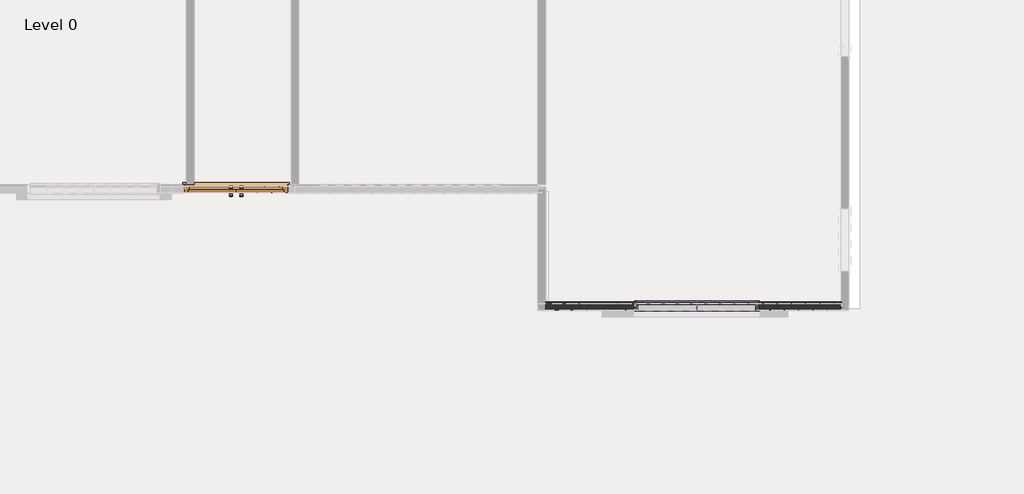
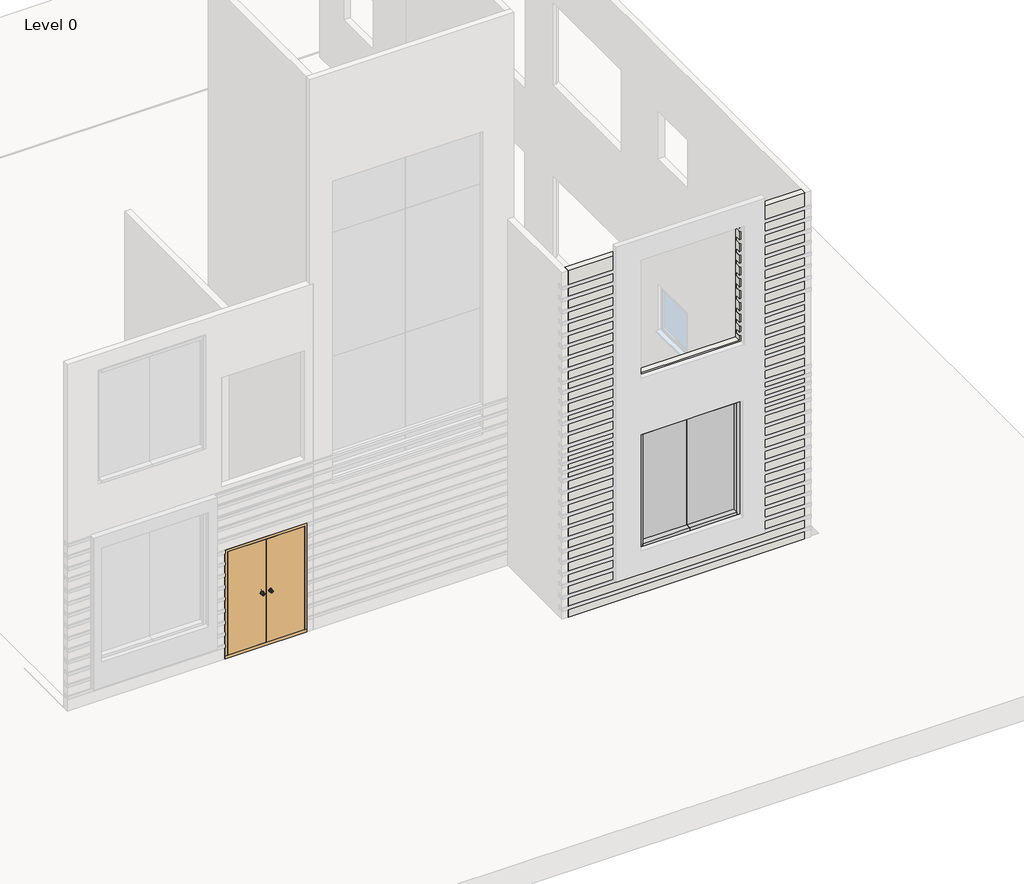
# One storey, part 2 of 5: 6 members, 2 plates, 1 door, 1 wall.
"""IFC4 building model written with IfcOpenShell, lengths in millimetres."""

from ifc_helpers import new_model, si_unit, origin, place, context, project, spatial, faceted_brep, transform, mapped, element, save
from components import doors_extdbl_flush_1510x2110mm_6aadbff8, rectangular_mullion_50x150mm_8753fc4c, rectangular_mullion_50x150mm_5ffedf64, system_panel_glazed_c09e287b

model = new_model("IFC4")

# Units and contexts
model_context = context("Model", 3, world=origin())
ifc_project = project(units=[si_unit("LENGTHUNIT", "METRE", prefix="MILLI")], contexts=[model_context])

# Site, building, storey
site = spatial("IfcSite", under=ifc_project)
building = spatial("IfcBuilding", under=site)
storey = spatial("IfcBuildingStorey", under=building, Name="Level 0", Elevation=0.0)

# Door
placement = place(None, origin())
doors_extdbl_flush_1510x2110mm_shape = doors_extdbl_flush_1510x2110mm_6aadbff8(model_context)
element("IfcDoor", 1, ObjectType="Doors_ExtDbl_Flush : 1510x2110mm", at=placement, inside=storey, context=model_context, shape_type="MappedRepresentation", body=[
    mapped(doors_extdbl_flush_1510x2110mm_shape, transform((-15773.529089, -2815.8968048, 0.0), x_axis=(1.0, 0.0, 0.0), y_axis=(0.0, 1.0, 0.0), z_axis=(0.0, 0.0, 1.0))),
])

# Members
rectangular_mullion_50x150mm_shape = rectangular_mullion_50x150mm_8753fc4c(model_context)
element("IfcMember", 2, ObjectType="Rectangular Mullion : 50x150mm", at=placement, inside=storey, context=model_context, shape_type="MappedRepresentation", body=[
    mapped(rectangular_mullion_50x150mm_shape, transform((-9930.929089, -4536.7468048, 3133.7021954), x_axis=(-1.0, 0.0, 0.0), y_axis=(0.0, -1.0, 0.0), z_axis=(0.0, 0.0, 1.0))),
])
element("IfcMember", 3, ObjectType="Rectangular Mullion : 50x150mm", at=placement, inside=storey, context=model_context, shape_type="MappedRepresentation", body=[
    mapped(rectangular_mullion_50x150mm_shape, transform((-8102.129089, -4536.7468048, 914.4), x_axis=(1.0, 0.0, 0.0), y_axis=(0.0, -1.0, 0.0), z_axis=(0.0, 0.0, -1.0))),
])
rectangular_mullion_50x150mm_2_shape = rectangular_mullion_50x150mm_5ffedf64(model_context)
element("IfcMember", 4, ObjectType="Rectangular Mullion : 50x150mm", at=placement, inside=storey, context=model_context, shape_type="MappedRepresentation", body=[
    mapped(rectangular_mullion_50x150mm_2_shape, transform((-8152.129089, -4536.7468048, 3133.7021954), x_axis=(0.0, 0.0, 1.0), y_axis=(0.0, -1.0, 0.0), z_axis=(1.0, 0.0, 0.0))),
])
element("IfcMember", 5, ObjectType="Rectangular Mullion : 50x150mm", at=placement, inside=storey, context=model_context, shape_type="MappedRepresentation", body=[
    mapped(rectangular_mullion_50x150mm_2_shape, transform((-9880.929089, -4536.7468048, 914.4), x_axis=(0.0, 0.0, -1.0), y_axis=(0.0, -1.0, 0.0), z_axis=(-1.0, 0.0, 0.0))),
])
element("IfcMember", 6, ObjectType="Rectangular Mullion : 50x150mm", at=placement, inside=storey, context=model_context, shape_type="MappedRepresentation", body=[
    mapped(rectangular_mullion_50x150mm_2_shape, transform((-9016.529089, -4536.7468048, 3133.7021954), x_axis=(0.0, 0.0, 1.0), y_axis=(0.0, -1.0, 0.0), z_axis=(1.0, 0.0, 0.0))),
])
element("IfcMember", 7, ObjectType="Rectangular Mullion : 50x150mm", at=placement, inside=storey, context=model_context, shape_type="MappedRepresentation", body=[
    mapped(rectangular_mullion_50x150mm_2_shape, transform((-9016.529089, -4536.7468048, 914.4), x_axis=(0.0, 0.0, -1.0), y_axis=(0.0, -1.0, 0.0), z_axis=(-1.0, 0.0, 0.0))),
])

# Plates
system_panel_glazed_shape = system_panel_glazed_c09e287b(model_context)
element("IfcPlate", 8, ObjectType="System Panel : Glazed", at=placement, inside=storey, context=model_context, shape_type="MappedRepresentation", body=[
    mapped(system_panel_glazed_shape, transform((-9448.729089, -4536.7468048, 964.4), x_axis=(1.0, 0.0, 0.0), y_axis=(0.0, 1.0, 0.0), z_axis=(0.0, 0.0, 1.0))),
])
element("IfcPlate", 9, ObjectType="System Panel : Glazed", at=placement, inside=storey, context=model_context, shape_type="MappedRepresentation", body=[
    mapped(system_panel_glazed_shape, transform((-8584.329089, -4536.7468048, 964.4), x_axis=(1.0, 0.0, 0.0), y_axis=(0.0, 1.0, 0.0), z_axis=(0.0, 0.0, 1.0))),
])

# Wall
element("IfcWall", 10, ObjectType="basic wall", at=placement, inside=storey, context=model_context, shape_type="Brep", body=[
    faceted_brep([(-11233.929089, -4593.8968048, 0.0), (-6903.229089, -4593.8968048, 0.0), (-6903.229089, -4593.8968048, 152.4), (-11233.929089, -4593.8968048, 152.4), (-6903.229089, -4593.8968048, 6705.6), (-11233.929089, -4593.8968048, 6705.6), (-11233.929089, -4593.8968048, 6439.3846362), (-9930.929089, -4593.8968048, 6439.3846362), (-9930.929089, -4593.8968048, 6486.5021954), (-8102.129089, -4593.8968048, 6486.5021954), (-8102.129089, -4593.8968048, 6439.3846362), (-6903.229089, -4593.8968048, 6439.3846362), (-9930.929089, -4593.8968048, 3133.7021954), (-8102.129089, -4593.8968048, 3133.7021954), (-8102.129089, -4593.8968048, 3193.5657622), (-6903.229089, -4593.8968048, 3193.5657622), (-6903.229089, -4593.8968048, 3290.2103724), (-11233.929089, -4593.8968048, 3290.2103724), (-11233.929089, -4593.8968048, 3193.5657622), (-9930.929089, -4593.8968048, 3193.5657622), (-8102.129089, -4593.8968048, 914.4), (-9930.929089, -4593.8968048, 914.4), (-9930.929089, -4593.8968048, 1059.0106439), (-11233.929089, -4593.8968048, 1059.0106439), (-11233.929089, -4593.8968048, 895.4106439), (-6903.229089, -4593.8968048, 895.4106439), (-6903.229089, -4593.8968048, 1059.0106439), (-8102.129089, -4593.8968048, 1059.0106439), (-8102.129089, -4593.8968048, 4267.2), (-9930.929089, -4593.8968048, 4267.2), (-9930.929089, -4593.8968048, 4358.4656265), (-11233.929089, -4593.8968048, 4358.4656265), (-11233.929089, -4593.8968048, 4202.6549826), (-6903.229089, -4593.8968048, 4202.6549826), (-6903.229089, -4593.8968048, 4358.4656265), (-8102.129089, -4593.8968048, 4358.4656265), (-11233.929089, -4593.8968048, 217.4), (-6903.229089, -4593.8968048, 217.4), (-6903.229089, -4593.8968048, 381.0), (-11233.929089, -4593.8968048, 381.0), (-11233.929089, -4593.8968048, 446.0), (-6903.229089, -4593.8968048, 446.0), (-6903.229089, -4593.8968048, 609.6), (-11233.929089, -4593.8968048, 609.6), (-11233.929089, -4593.8968048, 674.6), (-6903.229089, -4593.8968048, 674.6), (-6903.229089, -4593.8968048, 830.4106439), (-11233.929089, -4593.8968048, 830.4106439), (-8102.129089, -4593.8968048, 1124.0106439), (-6903.229089, -4593.8968048, 1124.0106439), (-6903.229089, -4593.8968048, 1279.8212878), (-8102.129089, -4593.8968048, 1279.8212878), (-11233.929089, -4593.8968048, 1124.0106439), (-9930.929089, -4593.8968048, 1124.0106439), (-9930.929089, -4593.8968048, 1279.8212878), (-11233.929089, -4593.8968048, 1279.8212878), (-8102.129089, -4593.8968048, 1344.8212878), (-6903.229089, -4593.8968048, 1344.8212878), (-6903.229089, -4593.8968048, 1500.6319317), (-8102.129089, -4593.8968048, 1500.6319317), (-11233.929089, -4593.8968048, 1344.8212878), (-9930.929089, -4593.8968048, 1344.8212878), (-9930.929089, -4593.8968048, 1500.6319317), (-11233.929089, -4593.8968048, 1500.6319317), (-8102.129089, -4593.8968048, 1565.6319317), (-6903.229089, -4593.8968048, 1565.6319317), (-6903.229089, -4593.8968048, 1729.2319317), (-8102.129089, -4593.8968048, 1729.2319317), (-11233.929089, -4593.8968048, 1565.6319317), (-9930.929089, -4593.8968048, 1565.6319317), (-9930.929089, -4593.8968048, 1729.2319317), (-11233.929089, -4593.8968048, 1729.2319317), (-8102.129089, -4593.8968048, 1794.2319317), (-6903.229089, -4593.8968048, 1794.2319317), (-6903.229089, -4593.8968048, 1957.8319317), (-8102.129089, -4593.8968048, 1957.8319317), (-11233.929089, -4593.8968048, 1794.2319317), (-9930.929089, -4593.8968048, 1794.2319317), (-9930.929089, -4593.8968048, 1957.8319317), (-11233.929089, -4593.8968048, 1957.8319317), (-8102.129089, -4593.8968048, 2022.8319317), (-6903.229089, -4593.8968048, 2022.8319317), (-6903.229089, -4593.8968048, 2186.4319317), (-8102.129089, -4593.8968048, 2186.4319317), (-11233.929089, -4593.8968048, 2022.8319317), (-9930.929089, -4593.8968048, 2022.8319317), (-9930.929089, -4593.8968048, 2186.4319317), (-11233.929089, -4593.8968048, 2186.4319317), (-8102.129089, -4593.8968048, 2251.4319317), (-6903.229089, -4593.8968048, 2251.4319317), (-6903.229089, -4593.8968048, 2415.0319317), (-8102.129089, -4593.8968048, 2415.0319317), (-11233.929089, -4593.8968048, 2251.4319317), (-9930.929089, -4593.8968048, 2251.4319317), (-9930.929089, -4593.8968048, 2415.0319317), (-11233.929089, -4593.8968048, 2415.0319317), (-8102.129089, -4593.8968048, 2480.0319317), (-6903.229089, -4593.8968048, 2480.0319317), (-6903.229089, -4593.8968048, 2643.6319317), (-8102.129089, -4593.8968048, 2643.6319317), (-11233.929089, -4593.8968048, 2480.0319317), (-9930.929089, -4593.8968048, 2480.0319317), (-9930.929089, -4593.8968048, 2643.6319317), (-11233.929089, -4593.8968048, 2643.6319317), (-8102.129089, -4593.8968048, 2708.6319317), (-6903.229089, -4593.8968048, 2708.6319317), (-6903.229089, -4593.8968048, 2805.2765418), (-8102.129089, -4593.8968048, 2805.2765418), (-11233.929089, -4593.8968048, 2708.6319317), (-9930.929089, -4593.8968048, 2708.6319317), (-9930.929089, -4593.8968048, 2805.2765418), (-11233.929089, -4593.8968048, 2805.2765418), (-8102.129089, -4593.8968048, 2870.2765418), (-6903.229089, -4593.8968048, 2870.2765418), (-6903.229089, -4593.8968048, 2966.921152), (-8102.129089, -4593.8968048, 2966.921152), (-11233.929089, -4593.8968048, 2870.2765418), (-9930.929089, -4593.8968048, 2870.2765418), (-9930.929089, -4593.8968048, 2966.921152), (-11233.929089, -4593.8968048, 2966.921152), (-8102.129089, -4593.8968048, 3031.921152), (-6903.229089, -4593.8968048, 3031.921152), (-6903.229089, -4593.8968048, 3128.5657622), (-8102.129089, -4593.8968048, 3128.5657622), (-11233.929089, -4593.8968048, 3031.921152), (-9930.929089, -4593.8968048, 3031.921152), (-9930.929089, -4593.8968048, 3128.5657622), (-11233.929089, -4593.8968048, 3128.5657622), (-11233.929089, -4593.8968048, 3355.2103724), (-6903.229089, -4593.8968048, 3355.2103724), (-6903.229089, -4593.8968048, 3518.8103724), (-11233.929089, -4593.8968048, 3518.8103724), (-11233.929089, -4593.8968048, 3583.8103724), (-6903.229089, -4593.8968048, 3583.8103724), (-6903.229089, -4593.8968048, 3747.4103724), (-11233.929089, -4593.8968048, 3747.4103724), (-11233.929089, -4593.8968048, 3812.4103724), (-6903.229089, -4593.8968048, 3812.4103724), (-6903.229089, -4593.8968048, 3909.0549826), (-11233.929089, -4593.8968048, 3909.0549826), (-11233.929089, -4593.8968048, 3974.0549826), (-6903.229089, -4593.8968048, 3974.0549826), (-6903.229089, -4593.8968048, 4137.6549826), (-11233.929089, -4593.8968048, 4137.6549826), (-8102.129089, -4593.8968048, 4423.4656265), (-6903.229089, -4593.8968048, 4423.4656265), (-6903.229089, -4593.8968048, 4545.5846362), (-8102.129089, -4593.8968048, 4545.5846362), (-11233.929089, -4593.8968048, 4423.4656265), (-9930.929089, -4593.8968048, 4423.4656265), (-9930.929089, -4593.8968048, 4545.5846362), (-11233.929089, -4593.8968048, 4545.5846362), (-8102.129089, -4593.8968048, 4610.5846362), (-6903.229089, -4593.8968048, 4610.5846362), (-6903.229089, -4593.8968048, 4774.1846362), (-8102.129089, -4593.8968048, 4774.1846362), (-11233.929089, -4593.8968048, 4610.5846362), (-9930.929089, -4593.8968048, 4610.5846362), (-9930.929089, -4593.8968048, 4774.1846362), (-11233.929089, -4593.8968048, 4774.1846362), (-8102.129089, -4593.8968048, 4839.1846362), (-6903.229089, -4593.8968048, 4839.1846362), (-6903.229089, -4593.8968048, 5002.7846362), (-8102.129089, -4593.8968048, 5002.7846362), (-11233.929089, -4593.8968048, 4839.1846362), (-9930.929089, -4593.8968048, 4839.1846362), (-9930.929089, -4593.8968048, 5002.7846362), (-11233.929089, -4593.8968048, 5002.7846362), (-8102.129089, -4593.8968048, 5067.7846362), (-6903.229089, -4593.8968048, 5067.7846362), (-6903.229089, -4593.8968048, 5231.3846362), (-8102.129089, -4593.8968048, 5231.3846362), (-11233.929089, -4593.8968048, 5067.7846362), (-9930.929089, -4593.8968048, 5067.7846362), (-9930.929089, -4593.8968048, 5231.3846362), (-11233.929089, -4593.8968048, 5231.3846362), (-8102.129089, -4593.8968048, 5296.3846362), (-6903.229089, -4593.8968048, 5296.3846362), (-6903.229089, -4593.8968048, 5459.9846362), (-8102.129089, -4593.8968048, 5459.9846362), (-11233.929089, -4593.8968048, 5296.3846362), (-9930.929089, -4593.8968048, 5296.3846362), (-9930.929089, -4593.8968048, 5459.9846362), (-11233.929089, -4593.8968048, 5459.9846362), (-8102.129089, -4593.8968048, 5524.9846362), (-6903.229089, -4593.8968048, 5524.9846362), (-6903.229089, -4593.8968048, 5688.5846362), (-8102.129089, -4593.8968048, 5688.5846362), (-11233.929089, -4593.8968048, 5524.9846362), (-9930.929089, -4593.8968048, 5524.9846362), (-9930.929089, -4593.8968048, 5688.5846362), (-11233.929089, -4593.8968048, 5688.5846362), (-8102.129089, -4593.8968048, 5753.5846362), (-6903.229089, -4593.8968048, 5753.5846362), (-6903.229089, -4593.8968048, 5917.1846362), (-8102.129089, -4593.8968048, 5917.1846362), (-11233.929089, -4593.8968048, 5753.5846362), (-9930.929089, -4593.8968048, 5753.5846362), (-9930.929089, -4593.8968048, 5917.1846362), (-11233.929089, -4593.8968048, 5917.1846362), (-8102.129089, -4593.8968048, 5982.1846362), (-6903.229089, -4593.8968048, 5982.1846362), (-6903.229089, -4593.8968048, 6145.7846362), (-8102.129089, -4593.8968048, 6145.7846362), (-11233.929089, -4593.8968048, 5982.1846362), (-9930.929089, -4593.8968048, 5982.1846362), (-9930.929089, -4593.8968048, 6145.7846362), (-11233.929089, -4593.8968048, 6145.7846362), (-8102.129089, -4593.8968048, 6210.7846362), (-6903.229089, -4593.8968048, 6210.7846362), (-6903.229089, -4593.8968048, 6374.3846362), (-8102.129089, -4593.8968048, 6374.3846362), (-11233.929089, -4593.8968048, 6210.7846362), (-9930.929089, -4593.8968048, 6210.7846362), (-9930.929089, -4593.8968048, 6374.3846362), (-11233.929089, -4593.8968048, 6374.3846362), (-6903.229089, -4479.5968048, 0.0), (-11233.929089, -4479.5968048, 0.0), (-11233.929089, -4479.5968048, 6705.6), (-6903.229089, -4479.5968048, 6705.6), (-9930.929089, -4479.5968048, 3133.7021954), (-9930.929089, -4479.5968048, 914.4), (-8102.129089, -4479.5968048, 914.4), (-8102.129089, -4479.5968048, 3133.7021954), (-9930.929089, -4479.5968048, 6486.5021954), (-9930.929089, -4479.5968048, 4267.2), (-8102.129089, -4479.5968048, 4267.2), (-8102.129089, -4479.5968048, 6486.5021954), (-11233.929089, -4501.3968048, 152.4), (-11233.929089, -4501.3968048, 227.4), (-11233.929089, -4583.8968048, 227.4), (-11233.929089, -4501.3968048, 381.0), (-11233.929089, -4501.3968048, 456.0), (-11233.929089, -4583.8968048, 456.0), (-11233.929089, -4501.3968048, 609.6), (-11233.929089, -4501.3968048, 684.6), (-11233.929089, -4583.8968048, 684.6), (-11233.929089, -4501.3968048, 830.4106439), (-11233.929089, -4501.3968048, 905.4106439), (-11233.929089, -4583.8968048, 905.4106439), (-11233.929089, -4501.3968048, 1059.0106439), (-11233.929089, -4501.3968048, 1134.0106439), (-11233.929089, -4583.8968048, 1134.0106439), (-11233.929089, -4501.3968048, 1279.8212878), (-11233.929089, -4501.3968048, 1354.8212878), (-11233.929089, -4583.8968048, 1354.8212878), (-11233.929089, -4501.3968048, 1500.6319317), (-11233.929089, -4501.3968048, 1575.6319317), (-11233.929089, -4583.8968048, 1575.6319317), (-11233.929089, -4501.3968048, 1729.2319317), (-11233.929089, -4501.3968048, 1804.2319317), (-11233.929089, -4583.8968048, 1804.2319317), (-11233.929089, -4501.3968048, 1957.8319317), (-11233.929089, -4501.3968048, 2032.8319317), (-11233.929089, -4583.8968048, 2032.8319317), (-11233.929089, -4501.3968048, 2186.4319317), (-11233.929089, -4501.3968048, 2261.4319317), (-11233.929089, -4583.8968048, 2261.4319317), (-11233.929089, -4501.3968048, 2415.0319317), (-11233.929089, -4501.3968048, 2490.0319317), (-11233.929089, -4583.8968048, 2490.0319317), (-11233.929089, -4501.3968048, 2643.6319317), (-11233.929089, -4501.3968048, 2718.6319317), (-11233.929089, -4583.8968048, 2718.6319317), (-11233.929089, -4501.3968048, 2805.2765418), (-11233.929089, -4501.3968048, 2880.2765418), (-11233.929089, -4583.8968048, 2880.2765418), (-11233.929089, -4501.3968048, 2966.921152), (-11233.929089, -4501.3968048, 3041.921152), (-11233.929089, -4583.8968048, 3041.921152), (-11233.929089, -4501.3968048, 3128.5657622), (-11233.929089, -4501.3968048, 3203.5657622), (-11233.929089, -4583.8968048, 3203.5657622), (-11233.929089, -4501.3968048, 3290.2103724), (-11233.929089, -4501.3968048, 3365.2103724), (-11233.929089, -4583.8968048, 3365.2103724), (-11233.929089, -4501.3968048, 3518.8103724), (-11233.929089, -4501.3968048, 3593.8103724), (-11233.929089, -4583.8968048, 3593.8103724), (-11233.929089, -4501.3968048, 3747.4103724), (-11233.929089, -4501.3968048, 3822.4103724), (-11233.929089, -4583.8968048, 3822.4103724), (-11233.929089, -4501.3968048, 3909.0549826), (-11233.929089, -4501.3968048, 3984.0549826), (-11233.929089, -4583.8968048, 3984.0549826), (-11233.929089, -4501.3968048, 4137.6549826), (-11233.929089, -4501.3968048, 4212.6549826), (-11233.929089, -4583.8968048, 4212.6549826), (-11233.929089, -4501.3968048, 4358.4656265), (-11233.929089, -4501.3968048, 4433.4656265), (-11233.929089, -4583.8968048, 4433.4656265), (-11233.929089, -4501.3968048, 4545.5846362), (-11233.929089, -4501.3968048, 4620.5846362), (-11233.929089, -4583.8968048, 4620.5846362), (-11233.929089, -4501.3968048, 4774.1846362), (-11233.929089, -4501.3968048, 4849.1846362), (-11233.929089, -4583.8968048, 4849.1846362), (-11233.929089, -4501.3968048, 5002.7846362), (-11233.929089, -4501.3968048, 5077.7846362), (-11233.929089, -4583.8968048, 5077.7846362), (-11233.929089, -4501.3968048, 5231.3846362), (-11233.929089, -4501.3968048, 5306.3846362), (-11233.929089, -4583.8968048, 5306.3846362), (-11233.929089, -4501.3968048, 5459.9846362), (-11233.929089, -4501.3968048, 5534.9846362), (-11233.929089, -4583.8968048, 5534.9846362), (-11233.929089, -4501.3968048, 5688.5846362), (-11233.929089, -4501.3968048, 5763.5846362), (-11233.929089, -4583.8968048, 5763.5846362), (-11233.929089, -4501.3968048, 5917.1846362), (-11233.929089, -4501.3968048, 5992.1846362), (-11233.929089, -4583.8968048, 5992.1846362), (-11233.929089, -4501.3968048, 6145.7846362), (-11233.929089, -4501.3968048, 6220.7846362), (-11233.929089, -4583.8968048, 6220.7846362), (-11233.929089, -4501.3968048, 6374.3846362), (-11233.929089, -4501.3968048, 6449.3846362), (-11233.929089, -4583.8968048, 6449.3846362), (-9930.929089, -4501.3968048, 3133.7021954), (-9930.929089, -4501.3968048, 3128.5657622), (-9930.929089, -4583.8968048, 3041.921152), (-9930.929089, -4501.3968048, 3041.921152), (-9930.929089, -4501.3968048, 2966.921152), (-9930.929089, -4583.8968048, 2880.2765418), (-9930.929089, -4501.3968048, 2880.2765418), (-9930.929089, -4501.3968048, 2805.2765418), (-9930.929089, -4583.8968048, 2718.6319317), (-9930.929089, -4501.3968048, 2718.6319317), (-9930.929089, -4501.3968048, 2643.6319317), (-9930.929089, -4583.8968048, 2490.0319317), (-9930.929089, -4501.3968048, 2490.0319317), (-9930.929089, -4501.3968048, 2415.0319317), (-9930.929089, -4583.8968048, 2261.4319317), (-9930.929089, -4501.3968048, 2261.4319317), (-9930.929089, -4501.3968048, 2186.4319317), (-9930.929089, -4583.8968048, 2032.8319317), (-9930.929089, -4501.3968048, 2032.8319317), (-9930.929089, -4501.3968048, 1957.8319317), (-9930.929089, -4583.8968048, 1804.2319317), (-9930.929089, -4501.3968048, 1804.2319317), (-9930.929089, -4501.3968048, 1729.2319317), (-9930.929089, -4583.8968048, 1575.6319317), (-9930.929089, -4501.3968048, 1575.6319317), (-9930.929089, -4501.3968048, 1500.6319317), (-9930.929089, -4583.8968048, 1354.8212878), (-9930.929089, -4501.3968048, 1354.8212878), (-9930.929089, -4501.3968048, 1279.8212878), (-9930.929089, -4583.8968048, 1134.0106439), (-9930.929089, -4501.3968048, 1134.0106439), (-9930.929089, -4501.3968048, 1059.0106439), (-8102.129089, -4501.3968048, 3133.7021954), (-8102.129089, -4501.3968048, 1059.0106439), (-8102.129089, -4501.3968048, 1134.0106439), (-8102.129089, -4583.8968048, 1134.0106439), (-8102.129089, -4501.3968048, 1279.8212878), (-8102.129089, -4501.3968048, 1354.8212878), (-8102.129089, -4583.8968048, 1354.8212878), (-8102.129089, -4501.3968048, 1500.6319317), (-8102.129089, -4501.3968048, 1575.6319317), (-8102.129089, -4583.8968048, 1575.6319317), (-8102.129089, -4501.3968048, 1729.2319317), (-8102.129089, -4501.3968048, 1804.2319317), (-8102.129089, -4583.8968048, 1804.2319317), (-8102.129089, -4501.3968048, 1957.8319317), (-8102.129089, -4501.3968048, 2032.8319317), (-8102.129089, -4583.8968048, 2032.8319317), (-8102.129089, -4501.3968048, 2186.4319317), (-8102.129089, -4501.3968048, 2261.4319317), (-8102.129089, -4583.8968048, 2261.4319317), (-8102.129089, -4501.3968048, 2415.0319317), (-8102.129089, -4501.3968048, 2490.0319317), (-8102.129089, -4583.8968048, 2490.0319317), (-8102.129089, -4501.3968048, 2643.6319317), (-8102.129089, -4501.3968048, 2718.6319317), (-8102.129089, -4583.8968048, 2718.6319317), (-8102.129089, -4501.3968048, 2805.2765418), (-8102.129089, -4501.3968048, 2880.2765418), (-8102.129089, -4583.8968048, 2880.2765418), (-8102.129089, -4501.3968048, 2966.921152), (-8102.129089, -4501.3968048, 3041.921152), (-8102.129089, -4583.8968048, 3041.921152), (-8102.129089, -4501.3968048, 3128.5657622), (-9930.929089, -4583.8968048, 6449.3846362), (-9930.929089, -4501.3968048, 6449.3846362), (-9930.929089, -4501.3968048, 6374.3846362), (-9930.929089, -4583.8968048, 6220.7846362), (-9930.929089, -4501.3968048, 6220.7846362), (-9930.929089, -4501.3968048, 6145.7846362), (-9930.929089, -4583.8968048, 5992.1846362), (-9930.929089, -4501.3968048, 5992.1846362), (-9930.929089, -4501.3968048, 5917.1846362), (-9930.929089, -4583.8968048, 5763.5846362), (-9930.929089, -4501.3968048, 5763.5846362), (-9930.929089, -4501.3968048, 5688.5846362), (-9930.929089, -4583.8968048, 5534.9846362), (-9930.929089, -4501.3968048, 5534.9846362), (-9930.929089, -4501.3968048, 5459.9846362), (-9930.929089, -4583.8968048, 5306.3846362), (-9930.929089, -4501.3968048, 5306.3846362), (-9930.929089, -4501.3968048, 5231.3846362), (-9930.929089, -4583.8968048, 5077.7846362), (-9930.929089, -4501.3968048, 5077.7846362), (-9930.929089, -4501.3968048, 5002.7846362), (-9930.929089, -4583.8968048, 4849.1846362), (-9930.929089, -4501.3968048, 4849.1846362), (-9930.929089, -4501.3968048, 4774.1846362), (-9930.929089, -4583.8968048, 4620.5846362), (-9930.929089, -4501.3968048, 4620.5846362), (-9930.929089, -4501.3968048, 4545.5846362), (-9930.929089, -4583.8968048, 4433.4656265), (-9930.929089, -4501.3968048, 4433.4656265), (-9930.929089, -4501.3968048, 4358.4656265), (-8102.129089, -4501.3968048, 4358.4656265), (-8102.129089, -4501.3968048, 4433.4656265), (-8102.129089, -4583.8968048, 4433.4656265), (-8102.129089, -4501.3968048, 4545.5846362), (-8102.129089, -4501.3968048, 4620.5846362), (-8102.129089, -4583.8968048, 4620.5846362), (-8102.129089, -4501.3968048, 4774.1846362), (-8102.129089, -4501.3968048, 4849.1846362), (-8102.129089, -4583.8968048, 4849.1846362), (-8102.129089, -4501.3968048, 5002.7846362), (-8102.129089, -4501.3968048, 5077.7846362), (-8102.129089, -4583.8968048, 5077.7846362), (-8102.129089, -4501.3968048, 5231.3846362), (-8102.129089, -4501.3968048, 5306.3846362), (-8102.129089, -4583.8968048, 5306.3846362), (-8102.129089, -4501.3968048, 5459.9846362), (-8102.129089, -4501.3968048, 5534.9846362), (-8102.129089, -4583.8968048, 5534.9846362), (-8102.129089, -4501.3968048, 5688.5846362), (-8102.129089, -4501.3968048, 5763.5846362), (-8102.129089, -4583.8968048, 5763.5846362), (-8102.129089, -4501.3968048, 5917.1846362), (-8102.129089, -4501.3968048, 5992.1846362), (-8102.129089, -4583.8968048, 5992.1846362), (-8102.129089, -4501.3968048, 6145.7846362), (-8102.129089, -4501.3968048, 6220.7846362), (-8102.129089, -4583.8968048, 6220.7846362), (-8102.129089, -4501.3968048, 6374.3846362), (-8102.129089, -4501.3968048, 6449.3846362), (-8102.129089, -4583.8968048, 6449.3846362), (-6903.229089, -4583.8968048, 6449.3846362), (-6903.229089, -4501.3968048, 6449.3846362), (-6903.229089, -4501.3968048, 6374.3846362), (-6903.229089, -4583.8968048, 6220.7846362), (-6903.229089, -4501.3968048, 6220.7846362), (-6903.229089, -4501.3968048, 6145.7846362), (-6903.229089, -4583.8968048, 5992.1846362), (-6903.229089, -4501.3968048, 5992.1846362), (-6903.229089, -4501.3968048, 5917.1846362), (-6903.229089, -4583.8968048, 5763.5846362), (-6903.229089, -4501.3968048, 5763.5846362), (-6903.229089, -4501.3968048, 5688.5846362), (-6903.229089, -4583.8968048, 5534.9846362), (-6903.229089, -4501.3968048, 5534.9846362), (-6903.229089, -4501.3968048, 5459.9846362), (-6903.229089, -4583.8968048, 5306.3846362), (-6903.229089, -4501.3968048, 5306.3846362), (-6903.229089, -4501.3968048, 5231.3846362), (-6903.229089, -4583.8968048, 5077.7846362), (-6903.229089, -4501.3968048, 5077.7846362), (-6903.229089, -4501.3968048, 5002.7846362), (-6903.229089, -4583.8968048, 4849.1846362), (-6903.229089, -4501.3968048, 4849.1846362), (-6903.229089, -4501.3968048, 4774.1846362), (-6903.229089, -4583.8968048, 4620.5846362), (-6903.229089, -4501.3968048, 4620.5846362), (-6903.229089, -4501.3968048, 4545.5846362), (-6903.229089, -4583.8968048, 4433.4656265), (-6903.229089, -4501.3968048, 4433.4656265), (-6903.229089, -4501.3968048, 4358.4656265), (-6903.229089, -4583.8968048, 4212.6549826), (-6903.229089, -4501.3968048, 4212.6549826), (-6903.229089, -4501.3968048, 4137.6549826), (-6903.229089, -4583.8968048, 3984.0549826), (-6903.229089, -4501.3968048, 3984.0549826), (-6903.229089, -4501.3968048, 3909.0549826), (-6903.229089, -4583.8968048, 3822.4103724), (-6903.229089, -4501.3968048, 3822.4103724), (-6903.229089, -4501.3968048, 3747.4103724), (-6903.229089, -4583.8968048, 3593.8103724), (-6903.229089, -4501.3968048, 3593.8103724), (-6903.229089, -4501.3968048, 3518.8103724), (-6903.229089, -4583.8968048, 3365.2103724), (-6903.229089, -4501.3968048, 3365.2103724), (-6903.229089, -4501.3968048, 3290.2103724), (-6903.229089, -4583.8968048, 3203.5657622), (-6903.229089, -4501.3968048, 3203.5657622), (-6903.229089, -4501.3968048, 3128.5657622), (-6903.229089, -4583.8968048, 3041.921152), (-6903.229089, -4501.3968048, 3041.921152), (-6903.229089, -4501.3968048, 2966.921152), (-6903.229089, -4583.8968048, 2880.2765418), (-6903.229089, -4501.3968048, 2880.2765418), (-6903.229089, -4501.3968048, 2805.2765418), (-6903.229089, -4583.8968048, 2718.6319317), (-6903.229089, -4501.3968048, 2718.6319317), (-6903.229089, -4501.3968048, 2643.6319317), (-6903.229089, -4583.8968048, 2490.0319317), (-6903.229089, -4501.3968048, 2490.0319317), (-6903.229089, -4501.3968048, 2415.0319317), (-6903.229089, -4583.8968048, 2261.4319317), (-6903.229089, -4501.3968048, 2261.4319317), (-6903.229089, -4501.3968048, 2186.4319317), (-6903.229089, -4583.8968048, 2032.8319317), (-6903.229089, -4501.3968048, 2032.8319317), (-6903.229089, -4501.3968048, 1957.8319317), (-6903.229089, -4583.8968048, 1804.2319317), (-6903.229089, -4501.3968048, 1804.2319317), (-6903.229089, -4501.3968048, 1729.2319317), (-6903.229089, -4583.8968048, 1575.6319317), (-6903.229089, -4501.3968048, 1575.6319317), (-6903.229089, -4501.3968048, 1500.6319317), (-6903.229089, -4583.8968048, 1354.8212878), (-6903.229089, -4501.3968048, 1354.8212878), (-6903.229089, -4501.3968048, 1279.8212878), (-6903.229089, -4583.8968048, 1134.0106439), (-6903.229089, -4501.3968048, 1134.0106439), (-6903.229089, -4501.3968048, 1059.0106439), (-6903.229089, -4583.8968048, 905.4106439), (-6903.229089, -4501.3968048, 905.4106439), (-6903.229089, -4501.3968048, 830.4106439), (-6903.229089, -4583.8968048, 684.6), (-6903.229089, -4501.3968048, 684.6), (-6903.229089, -4501.3968048, 609.6), (-6903.229089, -4583.8968048, 456.0), (-6903.229089, -4501.3968048, 456.0), (-6903.229089, -4501.3968048, 381.0), (-6903.229089, -4583.8968048, 227.4), (-6903.229089, -4501.3968048, 227.4), (-6903.229089, -4501.3968048, 152.4), (-8102.129089, -4501.3968048, 3203.5657622), (-8102.129089, -4583.8968048, 3203.5657622), (-9930.929089, -4583.8968048, 3203.5657622), (-9930.929089, -4501.3968048, 3203.5657622)], [[[0, 1, 2, 3]], [[4, 5, 6, 7, 8, 9, 10, 11]], [[12, 13, 14, 15, 16, 17, 18, 19]], [[20, 21, 22, 23, 24, 25, 26, 27]], [[28, 29, 30, 31, 32, 33, 34, 35]], [[36, 37, 38, 39]], [[40, 41, 42, 43]], [[44, 45, 46, 47]], [[48, 49, 50, 51]], [[52, 53, 54, 55]], [[56, 57, 58, 59]], [[60, 61, 62, 63]], [[64, 65, 66, 67]], [[68, 69, 70, 71]], [[72, 73, 74, 75]], [[76, 77, 78, 79]], [[80, 81, 82, 83]], [[84, 85, 86, 87]], [[88, 89, 90, 91]], [[92, 93, 94, 95]], [[96, 97, 98, 99]], [[100, 101, 102, 103]], [[104, 105, 106, 107]], [[108, 109, 110, 111]], [[112, 113, 114, 115]], [[116, 117, 118, 119]], [[120, 121, 122, 123]], [[124, 125, 126, 127]], [[128, 129, 130, 131]], [[132, 133, 134, 135]], [[136, 137, 138, 139]], [[140, 141, 142, 143]], [[144, 145, 146, 147]], [[148, 149, 150, 151]], [[152, 153, 154, 155]], [[156, 157, 158, 159]], [[160, 161, 162, 163]], [[164, 165, 166, 167]], [[168, 169, 170, 171]], [[172, 173, 174, 175]], [[176, 177, 178, 179]], [[180, 181, 182, 183]], [[184, 185, 186, 187]], [[188, 189, 190, 191]], [[192, 193, 194, 195]], [[196, 197, 198, 199]], [[200, 201, 202, 203]], [[204, 205, 206, 207]], [[208, 209, 210, 211]], [[212, 213, 214, 215]], [[216, 217, 218, 219], [220, 221, 222, 223], [224, 225, 226, 227]], [[1, 0, 217, 216]], [[5, 4, 219, 218]], [[5, 218, 217, 0, 3, 228, 229, 230, 36, 39, 231, 232, 233, 40, 43, 234, 235, 236, 44, 47, 237, 238, 239, 24, 23, 240, 241, 242, 52, 55, 243, 244, 245, 60, 63, 246, 247, 248, 68, 71, 249, 250, 251, 76, 79, 252, 253, 254, 84, 87, 255, 256, 257, 92, 95, 258, 259, 260, 100, 103, 261, 262, 263, 108, 111, 264, 265, 266, 116, 119, 267, 268, 269, 124, 127, 270, 271, 272, 18, 17, 273, 274, 275, 128, 131, 276, 277, 278, 132, 135, 279, 280, 281, 136, 139, 282, 283, 284, 140, 143, 285, 286, 287, 32, 31, 288, 289, 290, 148, 151, 291, 292, 293, 156, 159, 294, 295, 296, 164, 167, 297, 298, 299, 172, 175, 300, 301, 302, 180, 183, 303, 304, 305, 188, 191, 306, 307, 308, 196, 199, 309, 310, 311, 204, 207, 312, 313, 314, 212, 215, 315, 316, 317, 6]], [[21, 221, 220, 318, 319, 126, 125, 320, 321, 322, 118, 117, 323, 324, 325, 110, 109, 326, 327, 328, 102, 101, 329, 330, 331, 94, 93, 332, 333, 334, 86, 85, 335, 336, 337, 78, 77, 338, 339, 340, 70, 69, 341, 342, 343, 62, 61, 344, 345, 346, 54, 53, 347, 348, 349, 22]], [[13, 12, 318, 220, 223, 350]], [[222, 20, 27, 351, 352, 353, 48, 51, 354, 355, 356, 56, 59, 357, 358, 359, 64, 67, 360, 361, 362, 72, 75, 363, 364, 365, 80, 83, 366, 367, 368, 88, 91, 369, 370, 371, 96, 99, 372, 373, 374, 104, 107, 375, 376, 377, 112, 115, 378, 379, 380, 120, 123, 381, 350, 223]], [[221, 21, 20, 222]], [[29, 225, 224, 8, 7, 382, 383, 384, 214, 213, 385, 386, 387, 206, 205, 388, 389, 390, 198, 197, 391, 392, 393, 190, 189, 394, 395, 396, 182, 181, 397, 398, 399, 174, 173, 400, 401, 402, 166, 165, 403, 404, 405, 158, 157, 406, 407, 408, 150, 149, 409, 410, 411, 30]], [[8, 224, 227, 9]], [[9, 227, 226, 28, 35, 412, 413, 414, 144, 147, 415, 416, 417, 152, 155, 418, 419, 420, 160, 163, 421, 422, 423, 168, 171, 424, 425, 426, 176, 179, 427, 428, 429, 184, 187, 430, 431, 432, 192, 195, 433, 434, 435, 200, 203, 436, 437, 438, 208, 211, 439, 440, 441, 10]], [[225, 29, 28, 226]], [[1, 216, 219, 4, 11, 442, 443, 444, 210, 209, 445, 446, 447, 202, 201, 448, 449, 450, 194, 193, 451, 452, 453, 186, 185, 454, 455, 456, 178, 177, 457, 458, 459, 170, 169, 460, 461, 462, 162, 161, 463, 464, 465, 154, 153, 466, 467, 468, 146, 145, 469, 470, 471, 34, 33, 472, 473, 474, 142, 141, 475, 476, 477, 138, 137, 478, 479, 480, 134, 133, 481, 482, 483, 130, 129, 484, 485, 486, 16, 15, 487, 488, 489, 122, 121, 490, 491, 492, 114, 113, 493, 494, 495, 106, 105, 496, 497, 498, 98, 97, 499, 500, 501, 90, 89, 502, 503, 504, 82, 81, 505, 506, 507, 74, 73, 508, 509, 510, 66, 65, 511, 512, 513, 58, 57, 514, 515, 516, 50, 49, 517, 518, 519, 26, 25, 520, 521, 522, 46, 45, 523, 524, 525, 42, 41, 526, 527, 528, 38, 37, 529, 530, 531, 2]], [[531, 228, 3, 2]], [[230, 529, 37, 36]], [[529, 230, 229, 530]], [[228, 531, 530, 229]], [[528, 231, 39, 38]], [[233, 526, 41, 40]], [[526, 233, 232, 527]], [[231, 528, 527, 232]], [[525, 234, 43, 42]], [[236, 523, 45, 44]], [[523, 236, 235, 524]], [[234, 525, 524, 235]], [[522, 237, 47, 46]], [[239, 520, 25, 24]], [[520, 239, 238, 521]], [[237, 522, 521, 238]], [[519, 351, 27, 26]], [[353, 517, 49, 48]], [[517, 353, 352, 518]], [[351, 519, 518, 352]], [[349, 240, 23, 22]], [[242, 347, 53, 52]], [[347, 242, 241, 348]], [[240, 349, 348, 241]], [[516, 354, 51, 50]], [[356, 514, 57, 56]], [[514, 356, 355, 515]], [[354, 516, 515, 355]], [[346, 243, 55, 54]], [[245, 344, 61, 60]], [[344, 245, 244, 345]], [[243, 346, 345, 244]], [[513, 357, 59, 58]], [[359, 511, 65, 64]], [[511, 359, 358, 512]], [[357, 513, 512, 358]], [[343, 246, 63, 62]], [[248, 341, 69, 68]], [[341, 248, 247, 342]], [[246, 343, 342, 247]], [[510, 360, 67, 66]], [[362, 508, 73, 72]], [[508, 362, 361, 509]], [[360, 510, 509, 361]], [[340, 249, 71, 70]], [[251, 338, 77, 76]], [[338, 251, 250, 339]], [[249, 340, 339, 250]], [[507, 363, 75, 74]], [[365, 505, 81, 80]], [[505, 365, 364, 506]], [[363, 507, 506, 364]], [[337, 252, 79, 78]], [[254, 335, 85, 84]], [[335, 254, 253, 336]], [[252, 337, 336, 253]], [[504, 366, 83, 82]], [[368, 502, 89, 88]], [[502, 368, 367, 503]], [[366, 504, 503, 367]], [[334, 255, 87, 86]], [[257, 332, 93, 92]], [[332, 257, 256, 333]], [[255, 334, 333, 256]], [[501, 369, 91, 90]], [[371, 499, 97, 96]], [[499, 371, 370, 500]], [[369, 501, 500, 370]], [[331, 258, 95, 94]], [[260, 329, 101, 100]], [[329, 260, 259, 330]], [[258, 331, 330, 259]], [[498, 372, 99, 98]], [[374, 496, 105, 104]], [[496, 374, 373, 497]], [[372, 498, 497, 373]], [[328, 261, 103, 102]], [[263, 326, 109, 108]], [[326, 263, 262, 327]], [[261, 328, 327, 262]], [[495, 375, 107, 106]], [[377, 493, 113, 112]], [[493, 377, 376, 494]], [[375, 495, 494, 376]], [[325, 264, 111, 110]], [[266, 323, 117, 116]], [[323, 266, 265, 324]], [[264, 325, 324, 265]], [[492, 378, 115, 114]], [[380, 490, 121, 120]], [[490, 380, 379, 491]], [[378, 492, 491, 379]], [[322, 267, 119, 118]], [[269, 320, 125, 124]], [[320, 269, 268, 321]], [[267, 322, 321, 268]], [[532, 533, 14, 13, 350]], [[489, 381, 123, 122]], [[14, 533, 487, 15]], [[533, 532, 488, 487]], [[532, 350, 381, 489, 488]], [[534, 535, 318, 12, 19]], [[319, 270, 127, 126]], [[534, 19, 18, 272]], [[535, 534, 272, 271]], [[318, 535, 271, 270, 319]], [[486, 273, 17, 16]], [[275, 484, 129, 128]], [[484, 275, 274, 485]], [[273, 486, 485, 274]], [[483, 276, 131, 130]], [[278, 481, 133, 132]], [[481, 278, 277, 482]], [[276, 483, 482, 277]], [[480, 279, 135, 134]], [[281, 478, 137, 136]], [[478, 281, 280, 479]], [[279, 480, 479, 280]], [[477, 282, 139, 138]], [[284, 475, 141, 140]], [[475, 284, 283, 476]], [[282, 477, 476, 283]], [[474, 285, 143, 142]], [[287, 472, 33, 32]], [[472, 287, 286, 473]], [[285, 474, 473, 286]], [[471, 412, 35, 34]], [[414, 469, 145, 144]], [[469, 414, 413, 470]], [[412, 471, 470, 413]], [[411, 288, 31, 30]], [[290, 409, 149, 148]], [[409, 290, 289, 410]], [[288, 411, 410, 289]], [[468, 415, 147, 146]], [[417, 466, 153, 152]], [[466, 417, 416, 467]], [[415, 468, 467, 416]], [[408, 291, 151, 150]], [[293, 406, 157, 156]], [[406, 293, 292, 407]], [[291, 408, 407, 292]], [[465, 418, 155, 154]], [[420, 463, 161, 160]], [[463, 420, 419, 464]], [[418, 465, 464, 419]], [[405, 294, 159, 158]], [[296, 403, 165, 164]], [[403, 296, 295, 404]], [[294, 405, 404, 295]], [[462, 421, 163, 162]], [[423, 460, 169, 168]], [[460, 423, 422, 461]], [[421, 462, 461, 422]], [[402, 297, 167, 166]], [[299, 400, 173, 172]], [[400, 299, 298, 401]], [[297, 402, 401, 298]], [[459, 424, 171, 170]], [[426, 457, 177, 176]], [[457, 426, 425, 458]], [[424, 459, 458, 425]], [[399, 300, 175, 174]], [[302, 397, 181, 180]], [[397, 302, 301, 398]], [[300, 399, 398, 301]], [[456, 427, 179, 178]], [[429, 454, 185, 184]], [[454, 429, 428, 455]], [[427, 456, 455, 428]], [[396, 303, 183, 182]], [[305, 394, 189, 188]], [[394, 305, 304, 395]], [[303, 396, 395, 304]], [[453, 430, 187, 186]], [[432, 451, 193, 192]], [[451, 432, 431, 452]], [[430, 453, 452, 431]], [[393, 306, 191, 190]], [[308, 391, 197, 196]], [[391, 308, 307, 392]], [[306, 393, 392, 307]], [[450, 433, 195, 194]], [[435, 448, 201, 200]], [[448, 435, 434, 449]], [[433, 450, 449, 434]], [[390, 309, 199, 198]], [[311, 388, 205, 204]], [[388, 311, 310, 389]], [[309, 390, 389, 310]], [[447, 436, 203, 202]], [[438, 445, 209, 208]], [[445, 438, 437, 446]], [[436, 447, 446, 437]], [[387, 312, 207, 206]], [[314, 385, 213, 212]], [[385, 314, 313, 386]], [[312, 387, 386, 313]], [[444, 439, 211, 210]], [[441, 442, 11, 10]], [[442, 441, 440, 443]], [[439, 444, 443, 440]], [[384, 315, 215, 214]], [[317, 382, 7, 6]], [[382, 317, 316, 383]], [[315, 384, 383, 316]]]),
])

save(model, "model.ifc")

# Revit data of these elements
# Type "Doors_ExtDbl_Flush : 1510x2110mm"
#   Construction Type Id = "MDOOR"
#   Type Mark = "45"
#   Type Comments = "External Double"
#   Operation = "DoubleDoorSingleSwing"
#   Keynote = "L20"
#   Analytic Construction = "Metal"
#   Wrap Layers (Ext) from Ext = 0' - 4.03543"
#   Wrap Layers (Int) from Ext = 0' - 6.98819"
#   Thickness = 0' - 1.73228"
#   Rough Width = 4' - 11.44882"
#   Rough Height = 6' - 11.07087"
#   O/A Frame Width = 0' - 2.51969"
#   Heat Transfer Coefficient (U) = 3.7021 W/(m²·K)
#   Handle Z Distance = 3' - 5.33858"
#   FrameWidth = 0' - 1.65354"
#   FrameOffset - External = 0' - 0.98425"
#   FrameDepth = 0' - 3.50394"
#   Door Panel Width = 2' - 3.6378"
#   Door Panel Thickness = 0' - 1.73228"
#   Door Panel Height = 6' - 6.74016"
#   Cill Thickness = 0' - 2.14567"
#   Cill Projection = 0' - 1.1811"
#   Handle X Distance = 0' - 2.95276"
#   Height = 6' - 11.07087"
#   Structural Tolerance = 0' - 0.25591"
#   Tolerance = 0' - 0.11811"
#   Undercut = 0' - 0.15748"
#   Width = 4' - 11.44882"
#   Cill Extension = 0' - 0.98425"
#   Cavity Closer Width = 0' - 1.9685"
#   Cavity Closer Offset from Ext = 0' - 4.03543"
#   Cavity Closer Depth = 0' - 3.34646"
#   Define Thermal Properties by = 1
#   Vis - Ironmongery = yes
#   Vis - Cavity Closers = yes
#   Function = 1
#   Material Door = Door - Panel
#   Material Frame = Door - Frame/Mullion
#   Material Ironmongery = Door - Handle
#   Visual Light Transmittance = 0
#   Thermal Resistance (R) = 0
#   Solar Heat Gain Coefficient = 0
#   Wall Closure = (empty or 0)
# Type "Rectangular Mullion : 50x150mm"
#   Keynote = "H11"
#   built-in parameter 1007304 = 0.492126 (stored number, unit not read)
#   built-in parameter 1007301 = 0.082021 (stored number, unit not read)
#   built-in parameter 1007300 = 0.082021 (stored number, unit not read)
# Type "System Panel : Glazed"
#   Keynote = "H11"
#   Construction Type Id = "GSP4R"
#   Analytic Construction = "1/8 in Pilkington single glazing"
#   Visual Light Transmittance = 0.9
#   Solar Heat Gain Coefficient = 0.86
#   Heat Transfer Coefficient (U) = 6.7069 W/(m²·K)
#   Define Thermal Properties by = 1
# Type "basic wall"
#   Keynote = "F10"
#   Layers, outside or top first: 0' - 4 1/2" "Air" (function 1)
# Element 1 (IfcDoor, "Doors_ExtDbl_Flush : 1510x2110mm")
#   Phase Created = New Construction
#   Materials on its faces: "Door - Handle", "Door - Frame/Mullion", "Door - Panel"
# Elements 2, 3, 4, 5, 6, 7 (IfcMember, "Rectangular Mullion : 50x150mm")
#   Phase Created = New Construction
#   Materials on its faces: "Aluminium"
# Elements 8, 9 (IfcPlate, "System Panel : Glazed")
#   Phase Created = New Construction
#   Materials on its faces: "Glass"
# Element 10 (IfcWall, "basic wall")
#   Top Offset = 0' - 0"
#   Base Offset = 0' - 0"
#   wall height = 22' - 0"
#   Phase Created = New Construction
#   Base Constraint = Level 0
#   Top Constraint = Level 2
#   Materials on its faces: "Air"
# Materials
#   "Door - Panel": class "Wood", colour RGB 210 159 95, transparency 0, Keynote = "L20", Cost = 0
#   "Door - Frame/Mullion": class "Wood", colour RGB 212 179 113, transparency 0, Keynote = "L20", Cost = 0
#   "Door - Handle": colour RGB 17 17 17, transparency 0, Keynote = "P21", Cost = 0
#   "Air": class "Gas", colour RGB 255 255 255, transparency 0, Description = "Air", Cost = 0
#   "Aluminium": class "Metal", colour RGB 247 247 247, transparency 0, Description = "Aluminium 6061", Cost = 0
#   "Glass": class "Glass", colour RGB 0 128 192, transparency 0.9, Description = "Soda Lime Glass", Cost = 0
